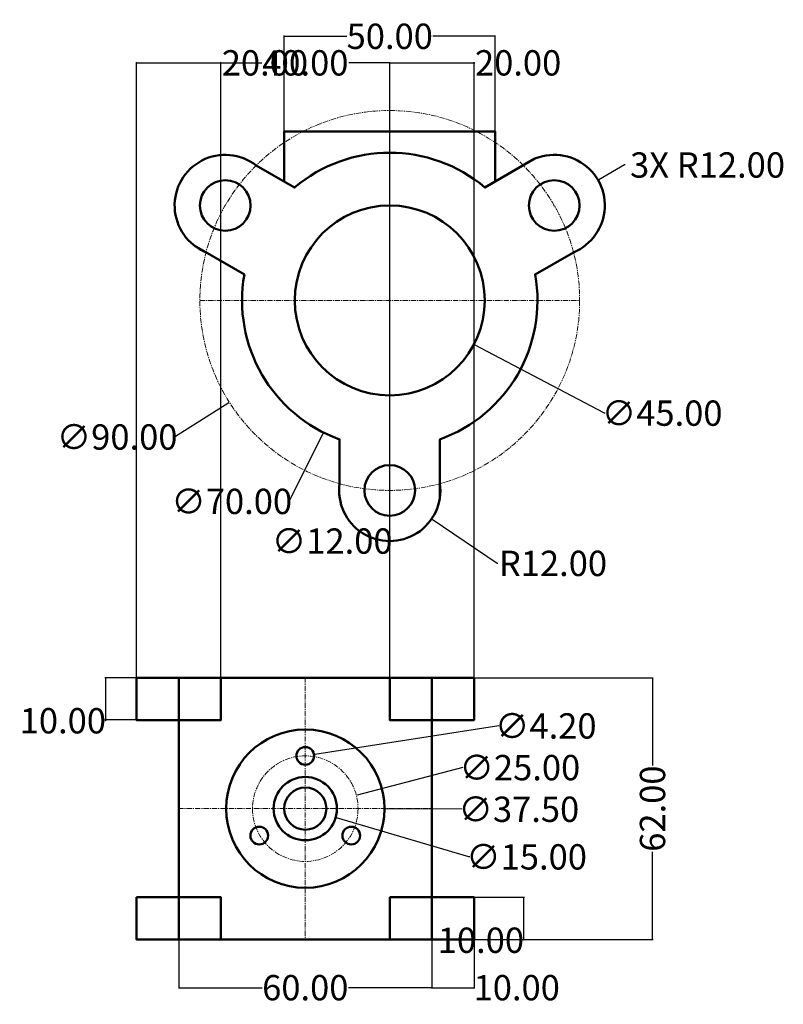
# Model space of a CAD drawing. Units: millimetres. Extents: x 0 to 181, y 8 to 241.
import ezdxf

# ---------------------------------------------------------------- set-up
doc = ezdxf.new("R2010")
doc.units = ezdxf.units.MM
doc.header["$MEASUREMENT"] = 0
doc.linetypes.add('CENTER', pattern=[2, 1.25, -0.25, 0.25, -0.25])
for name, color, linetype, lineweight in [('M-CNTR', 1, 'CENTER', 18), ('M-DIMS', 2, 'Continuous', 25), ('M-OUTL', 7, 'Continuous', 50)]:
    doc.layers.add(name, color=color, linetype=linetype, lineweight=lineweight)
doc.styles.get("Standard").update_dxf_attribs({"font": 'arial.ttf'})
doc.dimstyles.get("Standard").update_dxf_attribs({"dimtxt": 6, "dimasz": 0.18, "dimexe": 0.18, "dimexo": 0.0625, "dimgap": 0.09, "dimtad": 0, "dimtoh": 1, "dimzin": 0, "dimdsep": 46, "dimtxsty": 'Standard', "dimcen": 0.09, "dimadec": 0, "dimazin": 0, "dimtfac": 1, "dimtofl": 0, "dimtmove": 0, "dimatfit": 3, "dimfxl": 1, "dimtolj": 1, "dimtzin": 0, "dimarcsym": 0})

# ---------------------------------------------------------------- blocks, each defined once
blk = doc.blocks.new('*D1')
at = {"layer": 'Defpoints', "color": 0, "transparency": 16777216}
for p in [(112.37, 237.26), (62.37, 214.67), (112.37, 214.67)]:
    blk.add_point(p, dxfattribs=at)
at = {"layer": 'M-DIMS', "color": 0, "lineweight": -2, "transparency": 16777216}
for p, q in [((62.37, 214.74), (62.37, 237.44)), ((62.55, 237.26), (77.17, 237.26)), ((112.19, 237.26), (97.57, 237.26)), ((112.37, 214.74), (112.37, 237.44))]:
    blk.add_line(p, q, dxfattribs=at)
at = {"layer": 'M-DIMS', "color": 0, "transparency": 16777216}
for points in [[(62.55, 237.29), (62.55, 237.23), (62.37, 237.26)], [(112.19, 237.29), (112.19, 237.23), (112.37, 237.26)]]:
    blk.add_solid(points, dxfattribs=at)
at = {"layer": 'M-DIMS', "color": 0, "transparency": 16777216, "insert": (87.37, 237.26), "char_height": 6, "attachment_point": 5}
blk.add_mtext('\\A1;50.00', dxfattribs=at)
blk = doc.blocks.new('*D2')
at = {"layer": 'Defpoints', "color": 0, "transparency": 16777216}
for p in [(125.36, 198.79), (49.37, 150.56)]:
    blk.add_point(p, dxfattribs=at)
at = {"layer": 'M-DIMS', "color": 0, "lineweight": -2, "transparency": 16777216}
for p, q in [((87.28, 174.67), (87.46, 174.67)), ((87.37, 174.58), (87.37, 174.76)), ((36.4, 142.33), (49.22, 150.47)), ((36.22, 142.33), (36.4, 142.33))]:
    blk.add_line(p, q, dxfattribs=at)
at = {"layer": 'M-DIMS', "color": 0, "transparency": 16777216}
blk.add_solid([(49.21, 150.49), (49.24, 150.44), (49.37, 150.56)], dxfattribs=at)
at = {"layer": 'M-DIMS', "color": 0, "transparency": 16777216, "insert": (22.76, 142.33), "char_height": 6, "attachment_point": 5}
blk.add_mtext('\\A1;∅90.00', dxfattribs=at)
blk = doc.blocks.new('*D3')
at = {"layer": 'Defpoints', "color": 0, "transparency": 16777216}
for p in [(103.03, 205.98), (71.71, 143.37)]:
    blk.add_point(p, dxfattribs=at)
at = {"layer": 'M-DIMS', "color": 0, "lineweight": -2, "transparency": 16777216}
for p, q in [((87.28, 174.67), (87.46, 174.67)), ((87.37, 174.58), (87.37, 174.76)), ((63.56, 127.07), (71.63, 143.21)), ((63.38, 127.07), (63.56, 127.07))]:
    blk.add_line(p, q, dxfattribs=at)
at = {"layer": 'M-DIMS', "color": 0, "transparency": 16777216}
blk.add_solid([(71.61, 143.22), (71.66, 143.2), (71.71, 143.37)], dxfattribs=at)
at = {"layer": 'M-DIMS', "color": 0, "transparency": 16777216, "insert": (49.92, 127.07), "char_height": 6, "attachment_point": 5}
blk.add_mtext('\\A1;∅70.00', dxfattribs=at)
blk = doc.blocks.new('*D4')
at = {"layer": 'Defpoints', "color": 0, "transparency": 16777216}
for p in [(67.45, 185.13), (107.29, 164.22)]:
    blk.add_point(p, dxfattribs=at)
at = {"layer": 'M-DIMS', "color": 0, "lineweight": -2, "transparency": 16777216}
for p, q in [((87.28, 174.67), (87.46, 174.67)), ((87.37, 174.58), (87.37, 174.76)), ((138.25, 147.98), (107.45, 164.14)), ((138.43, 147.98), (138.25, 147.98))]:
    blk.add_line(p, q, dxfattribs=at)
at = {"layer": 'M-DIMS', "color": 0, "transparency": 16777216}
blk.add_solid([(107.47, 164.16), (107.44, 164.11), (107.29, 164.22)], dxfattribs=at)
at = {"layer": 'M-DIMS', "color": 0, "transparency": 16777216, "insert": (151.9, 147.98), "char_height": 6, "attachment_point": 5}
blk.add_mtext('\\A1;∅45.00', dxfattribs=at)
blk = doc.blocks.new('*D5')
at = {"layer": 'Defpoints', "color": 0, "transparency": 16777216}
for p in [(87.37, 135.67), (87.37, 123.67)]:
    blk.add_point(p, dxfattribs=at)
at = {"layer": 'M-DIMS', "color": 0, "lineweight": -2, "transparency": 16777216}
for p, q in [((87.28, 129.67), (87.46, 129.67)), ((87.37, 129.58), (87.37, 129.76)), ((87.37, 117.67), (87.37, 123.49)), ((87.19, 117.67), (87.37, 117.67))]:
    blk.add_line(p, q, dxfattribs=at)
at = {"layer": 'M-DIMS', "color": 0, "transparency": 16777216}
blk.add_solid([(87.34, 123.49), (87.4, 123.49), (87.37, 123.67)], dxfattribs=at)
at = {"layer": 'M-DIMS', "color": 0, "transparency": 16777216, "insert": (73.72, 117.67), "char_height": 6, "attachment_point": 5}
blk.add_mtext('\\A1;∅12.00', dxfattribs=at)
blk = doc.blocks.new('*D6')
at = {"layer": 'Defpoints', "color": 0, "transparency": 16777216}
for p in [(87.37, 129.67), (97.29, 122.92)]:
    blk.add_point(p, dxfattribs=at)
at = {"layer": 'M-DIMS', "color": 0, "lineweight": -2, "transparency": 16777216}
for p, q in [((87.28, 129.67), (87.46, 129.67)), ((87.37, 129.58), (87.37, 129.76)), ((112.79, 112.38), (97.44, 122.82)), ((112.97, 112.38), (112.79, 112.38))]:
    blk.add_line(p, q, dxfattribs=at)
at = {"layer": 'M-DIMS', "color": 0, "transparency": 16777216}
blk.add_solid([(97.46, 122.85), (97.42, 122.8), (97.29, 122.92)], dxfattribs=at)
at = {"layer": 'M-DIMS', "color": 0, "transparency": 16777216, "insert": (126.04, 112.38), "char_height": 6, "attachment_point": 5}
blk.add_mtext('\\A1;R12.00', dxfattribs=at)
blk = doc.blocks.new('*U7')
at = {"layer": 'M-CNTR', "color": 0, "transparency": 16777216}
blk.add_line((0, 31.12), (0, -31.12), dxfattribs=at)
blk = doc.blocks.new('*U8')
at = {"layer": 'M-CNTR', "color": 0, "transparency": 16777216}
blk.add_line((-30.12, 0), (30.12, 0), dxfattribs=at)
blk = doc.blocks.new('*D9')
at = {"layer": 'Defpoints', "color": 0, "transparency": 16777216}
for p in [(48.61, 54.35), (86.11, 54.21)]:
    blk.add_point(p, dxfattribs=at)
at = {"layer": 'M-DIMS', "color": 0, "lineweight": -2, "transparency": 16777216}
for p, q in [((67.27, 54.28), (67.45, 54.28)), ((67.36, 54.19), (67.36, 54.37)), ((104.49, 54.13), (86.29, 54.2))]:
    blk.add_line(p, q, dxfattribs=at)
at = {"layer": 'M-DIMS', "color": 0, "transparency": 16777216}
blk.add_solid([(86.29, 54.23), (86.29, 54.17), (86.11, 54.21)], dxfattribs=at)
at = {"layer": 'M-DIMS', "color": 0, "transparency": 16777216, "insert": (117.95, 54.13), "char_height": 6, "attachment_point": 5}
blk.add_mtext('\\A1;∅37.50', dxfattribs=at)
blk = doc.blocks.new('*D10')
at = {"layer": 'Defpoints', "color": 0, "transparency": 16777216}
for p in [(79.45, 57.43), (55.26, 51.13)]:
    blk.add_point(p, dxfattribs=at)
at = {"layer": 'M-DIMS', "color": 0, "lineweight": -2, "transparency": 16777216}
for p, q in [((104.72, 64), (79.63, 57.47)), ((67.27, 54.28), (67.45, 54.28)), ((67.36, 54.19), (67.36, 54.37))]:
    blk.add_line(p, q, dxfattribs=at)
at = {"layer": 'M-DIMS', "color": 0, "transparency": 16777216}
blk.add_solid([(79.62, 57.5), (79.64, 57.44), (79.45, 57.43)], dxfattribs=at)
at = {"layer": 'M-DIMS', "color": 0, "transparency": 16777216, "insert": (118.19, 64), "char_height": 6, "attachment_point": 5}
blk.add_mtext('\\A1;∅25.00', dxfattribs=at)
blk = doc.blocks.new('*D11')
at = {"layer": 'Defpoints', "color": 0, "transparency": 16777216}
for p in [(60.16, 56.4), (74.55, 52.16)]:
    blk.add_point(p, dxfattribs=at)
at = {"layer": 'M-DIMS', "color": 0, "lineweight": -2, "transparency": 16777216}
for p, q in [((67.27, 54.28), (67.45, 54.28)), ((67.36, 54.19), (67.36, 54.37)), ((106.13, 42.85), (74.72, 52.11)), ((106.31, 42.85), (106.13, 42.85))]:
    blk.add_line(p, q, dxfattribs=at)
at = {"layer": 'M-DIMS', "color": 0, "transparency": 16777216}
blk.add_solid([(74.73, 52.14), (74.72, 52.08), (74.55, 52.16)], dxfattribs=at)
at = {"layer": 'M-DIMS', "color": 0, "transparency": 16777216, "insert": (119.78, 42.85), "char_height": 6, "attachment_point": 5}
blk.add_mtext('\\A1;∅15.00', dxfattribs=at)
blk = doc.blocks.new('*D12')
at = {"layer": 'Defpoints', "color": 0, "transparency": 16777216}
for p in [(65.28, 66.46), (69.43, 67.1)]:
    blk.add_point(p, dxfattribs=at)
at = {"layer": 'M-DIMS', "color": 0, "lineweight": -2, "transparency": 16777216}
for p, q in [((113.19, 73.87), (69.61, 67.13)), ((67.27, 66.78), (67.45, 66.78)), ((67.36, 66.69), (67.36, 66.87))]:
    blk.add_line(p, q, dxfattribs=at)
at = {"layer": 'M-DIMS', "color": 0, "transparency": 16777216}
blk.add_solid([(69.61, 67.16), (69.62, 67.1), (69.43, 67.1)], dxfattribs=at)
at = {"layer": 'M-DIMS', "color": 0, "transparency": 16777216, "insert": (124.33, 73.87), "char_height": 6, "attachment_point": 5}
blk.add_mtext('\\A1;∅4.20', dxfattribs=at)
blk = doc.blocks.new('*D13')
at = {"layer": 'Defpoints', "color": 0, "transparency": 16777216}
for p in [(27.36, 85.28), (20.01, 75.28), (27.36, 75.28)]:
    blk.add_point(p, dxfattribs=at)
at = {"layer": 'M-DIMS', "color": 0, "lineweight": -2, "transparency": 16777216}
for p, q in [((27.3, 85.28), (19.83, 85.28)), ((20.01, 85.1), (20.01, 75.46)), ((27.3, 75.28), (19.83, 75.28)), ((20.01, 75.1), (19.83, 75.1)), ((20.01, 75.28), (20.01, 75.1))]:
    blk.add_line(p, q, dxfattribs=at)
at = {"layer": 'M-DIMS', "color": 0, "transparency": 16777216}
for points in [[(19.98, 85.1), (20.04, 85.1), (20.01, 85.28)], [(19.98, 75.46), (20.04, 75.46), (20.01, 75.28)]]:
    blk.add_solid(points, dxfattribs=at)
at = {"layer": 'M-DIMS', "color": 0, "transparency": 16777216, "insert": (9.91, 75.1), "char_height": 6, "attachment_point": 5}
blk.add_mtext('\\A1;10.00', dxfattribs=at)
blk = doc.blocks.new('*D14')
at = {"layer": 'Defpoints', "color": 0, "transparency": 16777216}
for p in [(107.36, 33.28), (107.36, 23.28), (119.08, 23.28)]:
    blk.add_point(p, dxfattribs=at)
at = {"layer": 'M-DIMS', "color": 0, "lineweight": -2, "transparency": 16777216}
for p, q in [((107.42, 33.28), (119.26, 33.28)), ((119.08, 33.1), (119.08, 23.46)), ((107.42, 23.28), (119.26, 23.28)), ((119.08, 23.1), (118.9, 23.1)), ((119.08, 23.28), (119.08, 23.1))]:
    blk.add_line(p, q, dxfattribs=at)
at = {"layer": 'M-DIMS', "color": 0, "transparency": 16777216}
for points in [[(119.05, 33.1), (119.11, 33.1), (119.08, 33.28)], [(119.05, 23.46), (119.11, 23.46), (119.08, 23.28)]]:
    blk.add_solid(points, dxfattribs=at)
at = {"layer": 'M-DIMS', "color": 0, "transparency": 16777216, "insert": (108.97, 23.1), "char_height": 6, "attachment_point": 5}
blk.add_mtext('\\A1;10.00', dxfattribs=at)
blk = doc.blocks.new('*D15')
at = {"layer": 'Defpoints', "color": 0, "transparency": 16777216}
for p in [(47.36, 230.97), (27.36, 85.28), (47.36, 85.28)]:
    blk.add_point(p, dxfattribs=at)
at = {"layer": 'M-DIMS', "color": 0, "lineweight": -2, "transparency": 16777216}
for p, q in [((27.36, 85.34), (27.36, 231.15)), ((27.54, 230.97), (47.18, 230.97)), ((47.36, 85.34), (47.36, 231.15)), ((47.36, 230.97), (47.54, 230.97))]:
    blk.add_line(p, q, dxfattribs=at)
at = {"layer": 'M-DIMS', "color": 0, "transparency": 16777216}
for points in [[(27.54, 231), (27.54, 230.94), (27.36, 230.97)], [(47.18, 231), (47.18, 230.94), (47.36, 230.97)]]:
    blk.add_solid(points, dxfattribs=at)
at = {"layer": 'M-DIMS', "color": 0, "transparency": 16777216, "insert": (57.79, 230.97), "char_height": 6, "attachment_point": 5}
blk.add_mtext('\\A1;20.00', dxfattribs=at)
blk = doc.blocks.new('*D16')
at = {"layer": 'Defpoints', "color": 0, "transparency": 16777216}
for p in [(87.36, 230.97), (47.36, 85.28), (87.36, 85.28)]:
    blk.add_point(p, dxfattribs=at)
at = {"layer": 'M-DIMS', "color": 0, "lineweight": -2, "transparency": 16777216}
for p, q in [((47.36, 85.34), (47.36, 231.15)), ((47.54, 230.97), (57.03, 230.97)), ((87.18, 230.97), (77.68, 230.97)), ((87.36, 85.34), (87.36, 231.15))]:
    blk.add_line(p, q, dxfattribs=at)
at = {"layer": 'M-DIMS', "color": 0, "transparency": 16777216}
for points in [[(47.54, 231), (47.54, 230.94), (47.36, 230.97)], [(87.18, 231), (87.18, 230.94), (87.36, 230.97)]]:
    blk.add_solid(points, dxfattribs=at)
at = {"layer": 'M-DIMS', "color": 0, "transparency": 16777216, "insert": (67.36, 230.97), "char_height": 6, "attachment_point": 5}
blk.add_mtext('\\A1;40.00', dxfattribs=at)
blk = doc.blocks.new('*D17')
at = {"layer": 'Defpoints', "color": 0, "transparency": 16777216}
for p in [(107.36, 230.97), (87.36, 85.28), (107.36, 85.28)]:
    blk.add_point(p, dxfattribs=at)
at = {"layer": 'M-DIMS', "color": 0, "lineweight": -2, "transparency": 16777216}
for p, q in [((87.36, 85.34), (87.36, 231.15)), ((87.54, 230.97), (107.18, 230.97)), ((107.36, 85.34), (107.36, 231.15)), ((107.36, 230.97), (107.54, 230.97))]:
    blk.add_line(p, q, dxfattribs=at)
at = {"layer": 'M-DIMS', "color": 0, "transparency": 16777216}
for points in [[(87.54, 231), (87.54, 230.94), (87.36, 230.97)], [(107.18, 231), (107.18, 230.94), (107.36, 230.97)]]:
    blk.add_solid(points, dxfattribs=at)
at = {"layer": 'M-DIMS', "color": 0, "transparency": 16777216, "insert": (117.79, 230.97), "char_height": 6, "attachment_point": 5}
blk.add_mtext('\\A1;20.00', dxfattribs=at)
blk = doc.blocks.new('*D18')
at = {"layer": 'Defpoints', "color": 0, "transparency": 16777216}
for p in [(37.36, 23.28), (97.36, 23.28), (97.36, 11.86)]:
    blk.add_point(p, dxfattribs=at)
at = {"layer": 'M-DIMS', "color": 0, "lineweight": -2, "transparency": 16777216}
for p, q in [((37.36, 23.22), (37.36, 11.68)), ((97.36, 23.22), (97.36, 11.68)), ((37.54, 11.86), (57.14, 11.86)), ((97.18, 11.86), (77.58, 11.86))]:
    blk.add_line(p, q, dxfattribs=at)
at = {"layer": 'M-DIMS', "color": 0, "transparency": 16777216}
for points in [[(37.54, 11.89), (37.54, 11.83), (37.36, 11.86)], [(97.18, 11.89), (97.18, 11.83), (97.36, 11.86)]]:
    blk.add_solid(points, dxfattribs=at)
at = {"layer": 'M-DIMS', "color": 0, "transparency": 16777216, "insert": (67.36, 11.86), "char_height": 6, "attachment_point": 5}
blk.add_mtext('\\A1;60.00', dxfattribs=at)
blk = doc.blocks.new('*D19')
at = {"layer": 'Defpoints', "color": 0, "transparency": 16777216}
for p in [(97.36, 23.28), (107.36, 23.28), (107.36, 11.86)]:
    blk.add_point(p, dxfattribs=at)
at = {"layer": 'M-DIMS', "color": 0, "lineweight": -2, "transparency": 16777216}
for p, q in [((97.36, 23.22), (97.36, 11.68)), ((107.36, 23.22), (107.36, 11.68)), ((97.54, 11.86), (107.18, 11.86)), ((107.36, 11.86), (107.54, 11.86))]:
    blk.add_line(p, q, dxfattribs=at)
at = {"layer": 'M-DIMS', "color": 0, "transparency": 16777216}
for points in [[(97.54, 11.89), (97.54, 11.83), (97.36, 11.86)], [(107.18, 11.89), (107.18, 11.83), (107.36, 11.86)]]:
    blk.add_solid(points, dxfattribs=at)
at = {"layer": 'M-DIMS', "color": 0, "transparency": 16777216, "insert": (117.46, 11.86), "char_height": 6, "attachment_point": 5}
blk.add_mtext('\\A1;10.00', dxfattribs=at)
blk = doc.blocks.new('*D20')
at = {"layer": 'Defpoints', "color": 0, "transparency": 16777216}
for p in [(97.36, 85.28), (149.63, 85.28), (97.36, 23.28)]:
    blk.add_point(p, dxfattribs=at)
at = {"layer": 'M-DIMS', "color": 0, "lineweight": -2, "transparency": 16777216}
for p, q in [((97.42, 85.28), (149.81, 85.28)), ((149.63, 85.1), (149.63, 64.5)), ((149.63, 23.46), (149.63, 44.06)), ((97.42, 23.28), (149.81, 23.28))]:
    blk.add_line(p, q, dxfattribs=at)
at = {"layer": 'M-DIMS', "color": 0, "transparency": 16777216}
for points in [[(149.6, 85.1), (149.66, 85.1), (149.63, 85.28)], [(149.6, 23.46), (149.66, 23.46), (149.63, 23.28)]]:
    blk.add_solid(points, dxfattribs=at)
at = {"layer": 'M-DIMS', "color": 0, "transparency": 16777216, "insert": (149.63, 54.28), "char_height": 6, "attachment_point": 5, "rotation": 90}
blk.add_mtext('\\A1;62.00', dxfattribs=at)
blk = doc.blocks.new('*D21')
at = {"layer": 'Defpoints', "color": 0, "transparency": 16777216}
for p in [(136.73, 203.17), (126.34, 197.17)]:
    blk.add_point(p, dxfattribs=at)
at = {"layer": 'M-DIMS', "color": 0, "lineweight": -2, "transparency": 16777216}
for p, q in [((142.97, 206.77), (136.89, 203.26)), ((143.15, 206.77), (142.97, 206.77)), ((126.25, 197.17), (126.43, 197.17)), ((126.34, 197.08), (126.34, 197.26))]:
    blk.add_line(p, q, dxfattribs=at)
at = {"layer": 'M-DIMS', "color": 0, "transparency": 16777216}
blk.add_solid([(136.87, 203.29), (136.9, 203.24), (136.73, 203.17)], dxfattribs=at)
at = {"layer": 'M-DIMS', "color": 0, "transparency": 16777216, "insert": (162.67, 206.77), "char_height": 6, "attachment_point": 5}
blk.add_mtext('\\A1;3X R12.00', dxfattribs=at)

msp = doc.modelspace()

# ---------------------------------------------------------------- linework, layer by layer
at = {"layer": 'M-CNTR'}
for p, q in [((87.37, 219.674), (87.37, 129.674)), ((42.37, 174.674), (132.37, 174.674))]:
    msp.add_line(p, q, dxfattribs=at)
for centre, radius in [((87.37, 174.674), 45), ((67.358, 54.278), 12.5)]:
    msp.add_circle(centre, radius, dxfattribs=at)
at = {"layer": 'M-OUTL'}
msp.add_lwpolyline([(112.37, 202.84), (112.37, 214.674), (87.37, 214.674), (87.37, 214.674), (62.37, 214.674), (62.37, 202.84)], dxfattribs=at)
for points in [[(121.78, 208.273), (109.931, 201.432, 0.3653105), (64.809, 201.432), (55.731, 206.673, 1.1435437), (43.838, 186.074)], [(119.009, 206.673, -1.1435437), (130.902, 186.074), (121.823, 180.833, -0.3653105), (99.263, 141.756), (99.263, 128.074)], [(41.066, 187.674), (52.916, 180.833, 0.3653105), (75.477, 141.756), (75.477, 131.274, 1.1435437), (99.263, 131.274)]]:
    msp.add_lwpolyline(points, format="xyb", dxfattribs=at)
for points in [[(27.358, 85.278), (27.358, 75.278), (47.358, 75.278), (47.358, 85.278), (37.358, 85.278)], [(37.358, 23.278), (97.358, 23.278), (97.358, 85.278), (37.358, 85.278)], [(87.358, 85.278), (87.358, 75.278), (107.358, 75.278), (107.358, 85.278), (97.358, 85.278)], [(27.358, 33.278), (27.358, 23.278), (47.358, 23.278), (47.358, 33.278), (37.358, 33.278)], [(87.358, 33.278), (87.358, 23.278), (107.358, 23.278), (107.358, 33.278), (97.358, 33.278)]]:
    msp.add_lwpolyline(points, close=True, dxfattribs=at)
for centre, radius in [((48.399, 197.174), 6), ((126.341, 197.174), 6), ((87.37, 174.674), 22.5), ((87.37, 129.674), 6), ((67.358, 54.278), 18.75), ((67.358, 66.778), 2.1), ((67.358, 54.278), 7.5), ((67.358, 54.278), 5), ((56.455, 47.893), 2.1), ((78.261, 47.893), 2.1)]:
    msp.add_circle(centre, radius, dxfattribs=at)

# ---------------------------------------------------------------- block references
at = {"layer": 'M-CNTR'}
for name in ['*U7', '*U8']:
    msp.add_blockref(name, (67.358, 54.278), dxfattribs=at)

# ---------------------------------------------------------------- dimensions: what is measured, and where the dimension line sits
at = {"layer": 'M-DIMS'}
for base, p1, p2, override, picture, middle in [((112.37, 237.259), (62.37, 214.674), (112.37, 214.674), {"dimclrd": 0, "dimclre": 0, "dimclrt": 0}, '*D1', (87.37, 237.259)), ((47.358, 230.974), (27.358, 85.278), (47.358, 85.278), {"dimdec": 2, "dimlfac": 1, "dimrnd": 0, "dimzin": 0, "dimdsep": 46, "dimlunit": 2}, '*D15', (57.792, 230.974)), ((87.358, 230.974), (47.358, 85.278), (87.358, 85.278), {"dimdec": 2, "dimlfac": 1, "dimrnd": 0, "dimzin": 0, "dimdsep": 46, "dimlunit": 2}, '*D16', (67.358, 230.974)), ((107.358, 230.974), (87.358, 85.278), (107.358, 85.278), {"dimdec": 2, "dimlfac": 1, "dimrnd": 0, "dimzin": 0, "dimdsep": 46, "dimlunit": 2}, '*D17', (117.792, 230.974)), ((97.358, 11.858), (37.358, 23.278), (97.358, 23.278), {"dimdec": 2, "dimlfac": 1, "dimrnd": 0, "dimzin": 0, "dimdsep": 46, "dimlunit": 2}, '*D18', (67.358, 11.858)), ((107.358, 11.858), (97.358, 23.278), (107.358, 23.278), {"dimdec": 2, "dimlfac": 1, "dimrnd": 0, "dimzin": 0, "dimdsep": 46, "dimlunit": 2}, '*D19', (117.459, 11.858))]:
    dim = msp.add_linear_dim(base=base, p1=p1, p2=p2, dimstyle='Standard', override=override, dxfattribs=at)
    dim.commit()
    dim.dimension.update_dxf_attribs({"geometry": picture, "text_midpoint": middle})
dim = msp.add_radius_dim(center=(126.341, 197.174), mpoint=(136.733, 203.174), text='3X <>', dimstyle='Standard', override={"dimdec": 2, "dimlfac": 1, "dimrnd": 0, "dimzin": 0, "dimdsep": 46, "dimlunit": 2}, dxfattribs=at)
dim.commit()
dim.dimension.update_dxf_attribs({"geometry": '*D21', "text_midpoint": (162.667, 206.774), "dimtype": 164})
for p1, p2, picture, middle in [((103.026, 205.977), (71.714, 143.371), '*D3', (49.915, 127.074)), ((125.365, 198.786), (49.375, 150.562), '*D2', (22.756, 142.33)), ((67.445, 185.127), (107.294, 164.221), '*D4', (151.899, 147.98)), ((87.37, 135.674), (87.37, 123.674), '*D5', (73.722, 117.674)), ((65.283, 66.457), (69.433, 67.1), '*D12', (113.193, 73.872)), ((55.261, 51.13), (79.455, 57.427), '*D10', (104.722, 64.003)), ((48.608, 54.351), (86.108, 54.205), '*D9', (104.487, 54.134)), ((60.164, 56.398), (74.552, 52.159), '*D11', (119.781, 42.855))]:
    dim = msp.add_diameter_dim_2p(p1=p1, p2=p2, dimstyle='Standard', override={"dimclrd": 0, "dimclre": 0, "dimclrt": 0}, dxfattribs=at)
    dim.commit()
    dim.dimension.update_dxf_attribs({"geometry": picture, "text_midpoint": middle, "dimtype": 163})
dim = msp.add_radius_dim(center=(87.37, 129.674), mpoint=(97.292, 122.925), dimstyle='Standard', override={"dimclrd": 0, "dimclre": 0, "dimclrt": 0}, dxfattribs=at)
dim.commit()
dim.dimension.update_dxf_attribs({"geometry": '*D6', "text_midpoint": (126.044, 112.382), "dimtype": 164})
for base, p1, p2, override, picture, middle in [((20.012, 75.278), (27.358, 85.278), (27.358, 75.278), {"dimclrd": 0, "dimclre": 0, "dimclrt": 0}, '*D13', (9.911, 75.098)), ((149.629, 85.278), (97.358, 23.278), (97.358, 85.278), {"dimdec": 2, "dimlfac": 1, "dimrnd": 0, "dimzin": 0, "dimdsep": 46, "dimlunit": 2}, '*D20', (149.629, 54.278)), ((119.076, 23.278), (107.358, 33.278), (107.358, 23.278), {"dimclrd": 0, "dimclre": 0, "dimclrt": 0}, '*D14', (108.975, 23.098))]:
    dim = msp.add_linear_dim(base=base, p1=p1, p2=p2, angle=90, dimstyle='Standard', override=override, dxfattribs=at)
    dim.commit()
    dim.dimension.update_dxf_attribs({"geometry": picture, "text_midpoint": middle})

doc.saveas('drawing.dxf')
